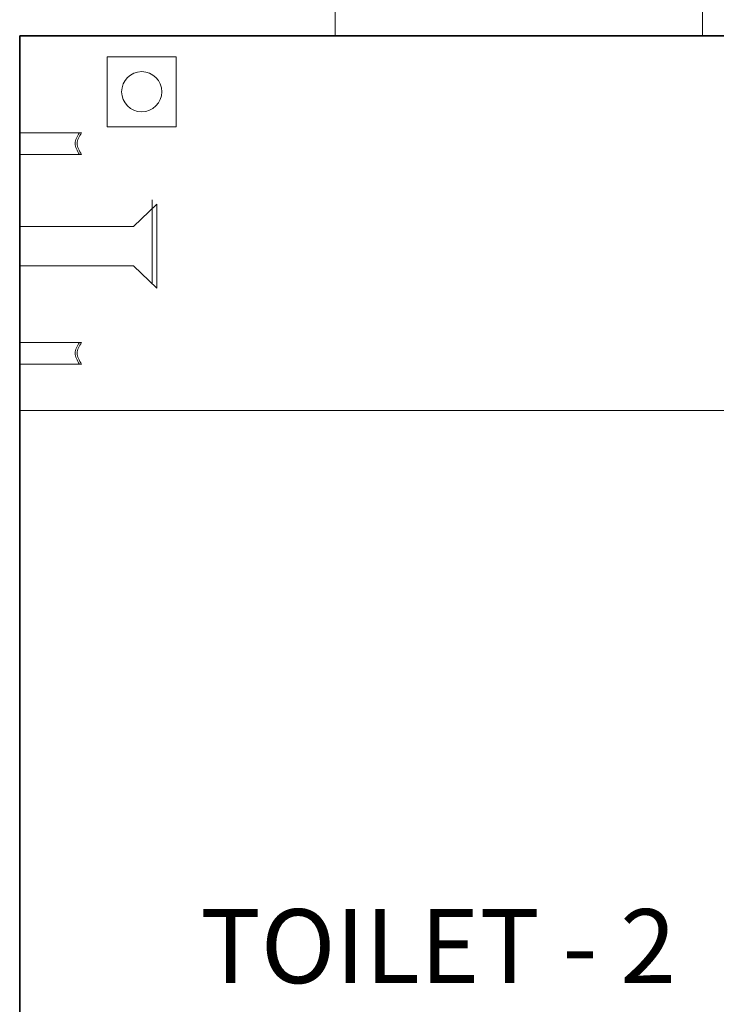
# Model space of a CAD drawing. Units: inches. Extents: x -61 to 1599, y -1316 to 257.
# Tile 173 of 204: x 1306 to 1351, y -684 to -620. Entities that reach past the tile are written whole.
import ezdxf

# ---------------------------------------------------------------- set-up
doc = ezdxf.new("R2010")
doc.units = ezdxf.units.IN
doc.header["$MEASUREMENT"] = 0
for name, color, linetype, lineweight in [('A-AREA-IDEN', 1, 'Continuous', 18), ('A-FLOR-FIXT', 8, 'Continuous', 18), ('WALLS', 4, 'Continuous', 35), ('WINDOWS', 220, 'Continuous', 18)]:
    doc.layers.add(name, color=color, linetype=linetype, lineweight=lineweight)
doc.styles.get("Standard").update_dxf_attribs({"font": 'arial.ttf'})

# ---------------------------------------------------------------- blocks, each defined once
blk = doc.blocks.new('WIN-24IN')
for p, q in [((0, 4.5), (0, 9)), ((0, 9), (0, 0)), ((24, 9), (24, 0)), ((0, 5.192), (24, 5.192)), ((0, 4.5), (24, 4.5))]:
    blk.add_line(p, q)
blk = doc.blocks.new('SHOWER-FITTINGS-2')
for p, q in [((0, 15.11), (4.042, 15.11)), ((0, 13.693), (4.042, 13.693)), ((7.429, 8.977), (8.952, 10.45)), ((8.658, 10.735), (8.658, 5.241)), ((8.952, 10.45), (8.952, 4.957)), ((0, 8.977), (7.429, 8.977)), ((0, 6.429), (7.429, 6.429)), ((7.429, 6.429), (8.952, 4.957)), ((0, 1.417), (4.042, 1.417)), ((0, 0), (4.042, 0))]:
    blk.add_line(p, q)
blk.add_lwpolyline([(10.232, 15.504), (5.711, 15.504), (5.711, 20.076), (10.232, 20.076)], close=True)
blk.add_circle((7.972, 17.79), 1.313)
for points in [[(3.906, 15.11), (3.762, 14.88), (3.468, 14.41), (3.758, 13.935), (3.906, 13.693)], [(4.042, 15.11), (3.898, 14.88), (3.604, 14.41), (3.894, 13.935), (4.042, 13.693)], [(3.906, 1.417), (3.762, 1.187), (3.468, 0.717), (3.758, 0.242), (3.906, 0)], [(4.042, 1.417), (3.898, 1.187), (3.604, 0.717), (3.894, 0.242), (4.042, 0)]]:
    blk.add_open_spline(points, degree=3, knots=[0, 0, 0, 0, 0.7501, 1.532449, 1.532449, 1.532449, 1.532449])

msp = doc.modelspace()

# ---------------------------------------------------------------- linework, layer by layer
at = {"layer": 'A-FLOR-FIXT'}
msp.add_line((1305.7028, -645.6384), (1375.7028, -645.6384), dxfattribs=at)
at = {"layer": 'WALLS'}
for q in [(1305.7028, -723.169), (1375.7028, -621.169)]:
    msp.add_line((1305.7028, -621.169), q, dxfattribs=at)

# ---------------------------------------------------------------- block references
at = {"layer": 'A-FLOR-FIXT'}
msp.add_blockref('SHOWER-FITTINGS-2', (1305.703, -642.6091), dxfattribs=at)
at = {"layer": 'WINDOWS'}
msp.add_blockref('WIN-24IN', (1326.3196, -621.1691), dxfattribs=at)

# ---------------------------------------------------------------- texts
at = {"layer": 'A-AREA-IDEN'}
msp.add_text('TOILET - 2', height=4.8321, dxfattribs=at).set_placement((1317.5043, -683.0366))

doc.saveas('drawing.dxf')
